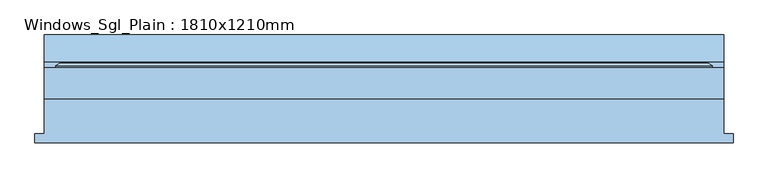
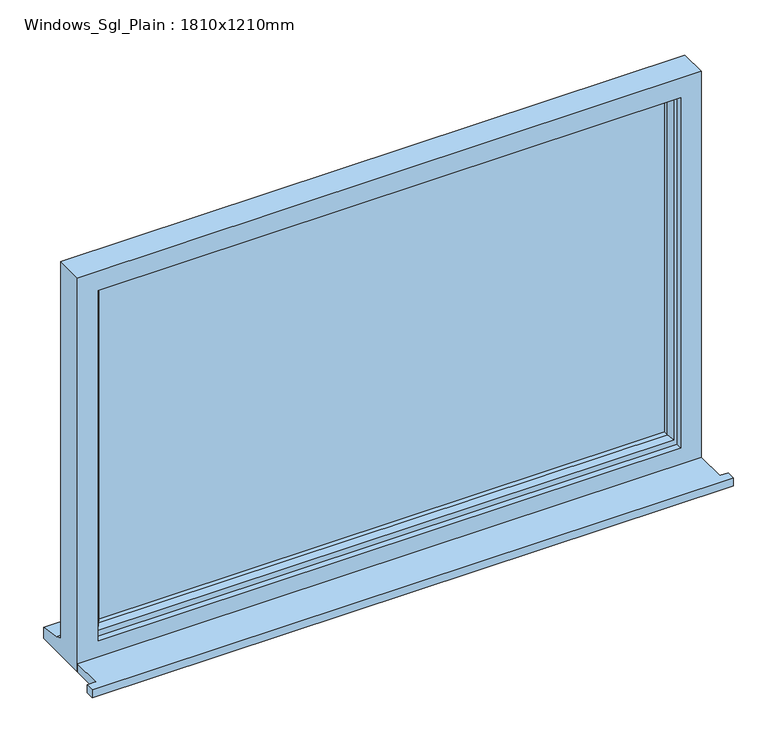
"""IFC4 building model written with IfcOpenShell, lengths in millimetres: window geometry, Windows_Sgl_Plain : 1810x1210mm."""

from ifc_helpers import new_model, si_unit, frame, origin, place, context, project, spatial, polyline, outline, extrude, faceted_brep, source, transform, mapped, element, save


def windows_sgl_plain_1810x1210mm_77c2169a(model_context):
    return source(origin(), model_context, "Body", "SolidModel", [
        extrude(outline(polyline([(-930.0, -129.0434322), (-930.0, -104.0434322), (-905.0, -104.0434322), (-905.0, -12.0434322), (905.0, -12.0434322), (905.0, -104.0434322), (930.0, -104.0434322), (930.0, -129.0434322), (-930.0, -129.0434322)])), frame((0.0, 0.0, 900.0), z_axis=(0.0, 0.0, 1.0), x_axis=(1.0, 0.0, 0.0)), (0.0, 0.0, 1.0), 25.0),
        faceted_brep([(-905.0, -12.0434322, 900.0), (905.0, -12.0434322, 900.0), (905.0, -12.0434322, 2110.0), (-905.0, -12.0434322, 2110.0), (-845.0, -12.0434322, 2050.0), (845.0, -12.0434322, 2050.0), (845.0, -12.0434322, 975.0), (-845.0, -12.0434322, 975.0), (-905.0, 70.9565678, 2110.0), (-905.0, 70.9565678, 951.0), (-905.0, 85.9565678, 949.68767), (-905.0, 85.9565678, 944.7449676), (-905.0, 158.4565678, 933.8088847), (-905.0, 158.4565678, 900.0), (905.0, 70.9565678, 2110.0), (905.0, 70.9565678, 951.0), (-865.0, 70.9565678, 2070.0), (-865.0, 70.9565678, 963.0), (865.0, 70.9565678, 963.0), (865.0, 70.9565678, 2070.0), (-865.0, 5.9565678, 2070.0), (-865.0, 5.9565678, 963.0), (865.0, 5.9565678, 2070.0), (865.0, 5.9565678, 963.0), (-845.0, 5.9565678, 2050.0), (-845.0, 5.9565678, 975.0), (845.0, 5.9565678, 975.0), (845.0, 5.9565678, 2050.0), (905.0, 158.4565678, 900.0), (905.0, 158.4565678, 933.8088847), (905.0, 85.9565678, 944.7449676), (905.0, 85.9565678, 949.68767)], [[[0, 1, 2, 3], [4, 5, 6, 7]], [[0, 3, 8, 9, 10, 11, 12, 13]], [[9, 8, 14, 15], [16, 17, 18, 19]], [[17, 16, 20, 21]], [[20, 22, 23, 21], [24, 25, 26, 27]], [[24, 4, 7, 25]], [[3, 2, 14, 8]], [[16, 19, 22, 20]], [[5, 4, 24, 27]], [[15, 14, 2, 1, 28, 29, 30, 31]], [[19, 18, 23, 22]], [[5, 27, 26, 6]], [[28, 1, 0, 13]], [[29, 28, 13, 12]], [[30, 29, 12, 11]], [[31, 30, 11, 10]], [[15, 31, 10, 9]], [[21, 23, 18, 17]], [[7, 6, 26, 25]]]),
        extrude(outline(polyline([(835.0, 34.9565678), (-835.0, 34.9565678), (-835.0, 58.9565678), (835.0, 58.9565678), (835.0, 34.9565678)])), frame((0.0, 0.0, 993.0), z_axis=(0.0, 0.0, 1.0), x_axis=(1.0, 0.0, 0.0)), (0.0, 0.0, 1.0), 1047.0),
        faceted_brep([(-875.0, 70.9565678, 2080.0), (-875.0, 76.7300705, 2080.0), (-875.0, 76.7300705, 953.0), (-875.0, 70.9565678, 953.0), (-865.0, 5.9565678, 2070.0), (-865.0, 70.9565678, 2070.0), (-865.0, 70.9565678, 963.0), (-865.0, 5.9565678, 963.0), (-825.0, 20.4494677, 2030.0), (-835.1480377, 5.9565678, 2040.1480377), (-835.1480377, 5.9565678, 992.8519623), (-825.0, 20.4494677, 1003.0), (-825.0, 34.9565678, 2030.0), (-825.0, 34.9565678, 1003.0), (-835.0, 58.9565678, 2040.0), (-835.0, 34.9565678, 2040.0), (-835.0, 34.9565678, 993.0), (-835.0, 58.9565678, 993.0), (-825.0, 76.7300705, 2030.0), (-825.0, 58.9565678, 2030.0), (-825.0, 58.9565678, 1003.0), (-825.0, 76.7300705, 1003.0), (-842.4457548, 82.5035732, 2047.4457548), (-842.4457548, 82.5035732, 985.5542452), (-864.2153903, 82.5035732, 2069.2153903), (-864.2153903, 82.5035732, 963.7846097), (875.0, 76.7300705, 953.0), (875.0, 70.9565678, 953.0), (865.0, 70.9565678, 963.0), (865.0, 5.9565678, 963.0), (835.1480377, 5.9565678, 992.8519623), (825.0, 20.4494677, 1003.0), (825.0, 34.9565678, 1003.0), (835.0, 34.9565678, 993.0), (835.0, 58.9565678, 993.0), (825.0, 58.9565678, 1003.0), (825.0, 76.7300705, 1003.0), (842.4457548, 82.5035732, 985.5542452), (864.2153903, 82.5035732, 963.7846097), (875.0, 76.7300705, 2080.0), (875.0, 70.9565678, 2080.0), (865.0, 70.9565678, 2070.0), (865.0, 5.9565678, 2070.0), (835.1480377, 5.9565678, 2040.1480377), (825.0, 20.4494677, 2030.0), (825.0, 34.9565678, 2030.0), (835.0, 34.9565678, 2040.0), (835.0, 58.9565678, 2040.0), (825.0, 58.9565678, 2030.0), (825.0, 76.7300705, 2030.0), (842.4457548, 82.5035732, 2047.4457548), (864.2153903, 82.5035732, 2069.2153903)], [[[0, 1, 2, 3]], [[4, 5, 6, 7]], [[8, 9, 10, 11]], [[12, 8, 11, 13]], [[14, 15, 16, 17]], [[18, 19, 20, 21]], [[22, 18, 21, 23]], [[1, 24, 25, 2]], [[3, 2, 26, 27]], [[7, 6, 28, 29]], [[11, 10, 30, 31]], [[13, 11, 31, 32]], [[17, 16, 33, 34]], [[21, 20, 35, 36]], [[23, 21, 36, 37]], [[2, 25, 38, 26]], [[27, 26, 39, 40]], [[29, 28, 41, 42]], [[31, 30, 43, 44]], [[32, 31, 44, 45]], [[34, 33, 46, 47]], [[36, 35, 48, 49]], [[37, 36, 49, 50]], [[26, 38, 51, 39]], [[40, 39, 1, 0]], [[3, 27, 40, 0], [5, 41, 28, 6]], [[42, 41, 5, 4]], [[7, 29, 42, 4], [9, 43, 30, 10]], [[44, 43, 9, 8]], [[45, 44, 8, 12]], [[15, 46, 33, 16], [13, 32, 45, 12]], [[47, 46, 15, 14]], [[17, 34, 47, 14], [19, 48, 35, 20]], [[49, 48, 19, 18]], [[50, 49, 18, 22]], [[24, 51, 38, 25], [23, 37, 50, 22]], [[39, 51, 24, 1]]]),
    ])


if __name__ == "__main__":
    model = new_model("IFC4")
    model_context = context("Model", 3, world=origin())
    ifc_project = project(units=[si_unit("LENGTHUNIT", "METRE", prefix="MILLI")], contexts=[model_context])
    site = spatial("IfcSite", under=ifc_project)
    building = spatial("IfcBuilding", under=site)
    placement = place(None, origin())
    windows_sgl_plain_1810x1210mm_shape = windows_sgl_plain_1810x1210mm_77c2169a(model_context)
    element("IfcWindow", 1, ObjectType="Windows_Sgl_Plain : 1810x1210mm", at=placement, inside=building, context=model_context, shape_type="MappedRepresentation", body=[
        mapped(windows_sgl_plain_1810x1210mm_shape, transform((0.0, 0.0, 0.0), x_axis=(1.0, 0.0, 0.0), y_axis=(0.0, 1.0, 0.0), z_axis=(0.0, 0.0, 1.0))),
    ])
    save(model, "model.ifc")

# Revit data of these elements
# Type "Windows_Sgl_Plain : 1810x1210mm"
#   Type Mark = "49"
#   Operation = "SinglePanel"
#   Construction Type Id = "SGL"
#   Manufacturer = "Revit"
#   Keynote = "L10"
#   Analytic Construction = "Large single-glazed windows"
#   Wrap Layers (Ext) from Ext = 102.5 mm
#   Wrap Layers (Int) from Ext = 177.5 mm
#   Window Board Projection = 25 mm
#   Window Board Extension = 25 mm
#   Visual Light Transmittance = 0.9
#   Solar Heat Gain Coefficient = 0.86
#   Rough Width = 1810 mm
#   Rough Height = 1210 mm
#   Height = 1210 mm
#   Width = 1810 mm
#   Heat Transfer Coefficient (U) = 5.5617 W/(m²·K)
#   Glazing Thickness = 24 mm
#   FrameOffset - External = 50 mm
#   Frame Depth = 65 mm
#   Default Head Height = 2110 mm
#   Cill Depth = 87.5 mm
#   Cavity Closer Width = 50 mm
#   Cavity Closer Offset from Ext = 102.5 mm
#   Cavity Closer Depth = 85 mm
#   Define Thermal Properties by = 1
#   Vis - Cavity Closers = yes
#   Define Thermal Properties by = 1
#   Material Trim = Window Frame
#   Material Glass = Glass
#   Material Frame = Window Frame
#   Wall Closure = (empty or 0)
# Element 1 (IfcWindow, "Windows_Sgl_Plain : 1810x1210mm")
#   Materials on its faces: "Window Frame", "Glass"
# Materials
#   "Window Frame": colour RGB 249 249 249, transparency 0, Keynote = "L10", Cost = 0
#   "Glass": class "Glass", colour RGB 0 128 192, transparency 0.9, Description = "Soda Lime Glass", Cost = 0
